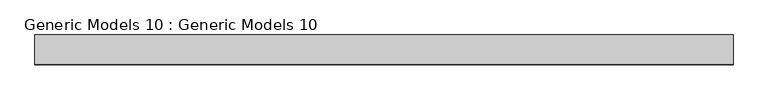
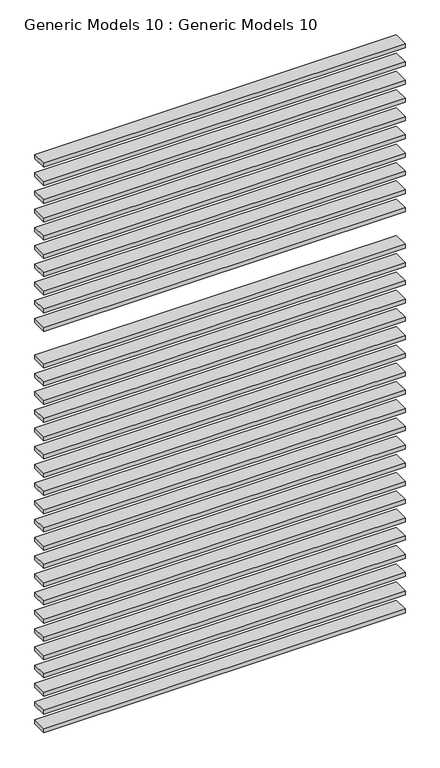
"""IFC4 building model written with IfcOpenShell, lengths in millimetres: proxy geometry, Generic Models 10 : Generic Models 10."""

from ifc_helpers import new_model, si_unit, frame, origin, place, context, project, spatial, polyline, outline, extrude, source, transform, mapped, element, save


def generic_models_10_generic_models_10_37b285cf(model_context):
    return source(origin(), model_context, "Body", "SweptSolid", [
        extrude(outline(polyline([(-8004.4916253, -6728.8336164), (-10858.4873516, -6728.8336164), (-10858.4873516, -6608.1640695), (-8004.4916253, -6608.1640695), (-8004.4916253, -6728.8336164)])), frame((0.0, 0.0, 3244.6584632), z_axis=(0.0, 0.0, 1.0), x_axis=(1.0, 0.0, 0.0)), (0.0, 0.0, 1.0), 33.1662923),
        extrude(outline(polyline([(-8004.4916253, -6728.8336164), (-10858.4873516, -6728.8336164), (-10858.4873516, -6608.1640695), (-8004.4916253, -6608.1640695), (-8004.4916253, -6728.8336164)])), frame((0.0, 0.0, 3397.0584632), z_axis=(0.0, 0.0, 1.0), x_axis=(1.0, 0.0, 0.0)), (0.0, 0.0, 1.0), 33.1662923),
        extrude(outline(polyline([(-8004.4916253, -6728.8336164), (-10858.4873516, -6728.8336164), (-10858.4873516, -6608.1640695), (-8004.4916253, -6608.1640695), (-8004.4916253, -6728.8336164)])), frame((0.0, 0.0, 3549.4584632), z_axis=(0.0, 0.0, 1.0), x_axis=(1.0, 0.0, 0.0)), (0.0, 0.0, 1.0), 33.1662923),
        extrude(outline(polyline([(-8004.4916253, -6728.8336164), (-10858.4873516, -6728.8336164), (-10858.4873516, -6608.1640695), (-8004.4916253, -6608.1640695), (-8004.4916253, -6728.8336164)])), frame((0.0, 0.0, 3701.8584632), z_axis=(0.0, 0.0, 1.0), x_axis=(1.0, 0.0, 0.0)), (0.0, 0.0, 1.0), 33.1662923),
        extrude(outline(polyline([(-8004.4916253, -6728.8336164), (-10858.4873516, -6728.8336164), (-10858.4873516, -6608.1640695), (-8004.4916253, -6608.1640695), (-8004.4916253, -6728.8336164)])), frame((0.0, 0.0, 3854.2584632), z_axis=(0.0, 0.0, 1.0), x_axis=(1.0, 0.0, 0.0)), (0.0, 0.0, 1.0), 33.1662923),
        extrude(outline(polyline([(-8004.4916253, -6728.8336164), (-10858.4873516, -6728.8336164), (-10858.4873516, -6608.1640695), (-8004.4916253, -6608.1640695), (-8004.4916253, -6728.8336164)])), frame((0.0, 0.0, 4006.6584632), z_axis=(0.0, 0.0, 1.0), x_axis=(1.0, 0.0, 0.0)), (0.0, 0.0, 1.0), 33.1662923),
        extrude(outline(polyline([(-8004.4916253, -6728.8336164), (-10858.4873516, -6728.8336164), (-10858.4873516, -6608.1640695), (-8004.4916253, -6608.1640695), (-8004.4916253, -6728.8336164)])), frame((0.0, 0.0, 4159.0584632), z_axis=(0.0, 0.0, 1.0), x_axis=(1.0, 0.0, 0.0)), (0.0, 0.0, 1.0), 33.1662923),
        extrude(outline(polyline([(-8004.4916253, -6728.8336164), (-10858.4873516, -6728.8336164), (-10858.4873516, -6608.1640695), (-8004.4916253, -6608.1640695), (-8004.4916253, -6728.8336164)])), frame((0.0, 0.0, 4311.4584632), z_axis=(0.0, 0.0, 1.0), x_axis=(1.0, 0.0, 0.0)), (0.0, 0.0, 1.0), 33.1662923),
        extrude(outline(polyline([(-8004.4916253, -6728.8336164), (-10858.4873516, -6728.8336164), (-10858.4873516, -6608.1640695), (-8004.4916253, -6608.1640695), (-8004.4916253, -6728.8336164)])), frame((0.0, 0.0, 4463.8584632), z_axis=(0.0, 0.0, 1.0), x_axis=(1.0, 0.0, 0.0)), (0.0, 0.0, 1.0), 33.1662923),
        extrude(outline(polyline([(-8004.4916253, -6728.8336164), (-10858.4873516, -6728.8336164), (-10858.4873516, -6608.1640695), (-8004.4916253, -6608.1640695), (-8004.4916253, -6728.8336164)])), frame((0.0, 0.0, 4616.2584632), z_axis=(0.0, 0.0, 1.0), x_axis=(1.0, 0.0, 0.0)), (0.0, 0.0, 1.0), 33.1662923),
        extrude(outline(polyline([(-8004.4916253, -6728.8336164), (-10858.4873516, -6728.8336164), (-10858.4873516, -6608.1640695), (-8004.4916253, -6608.1640695), (-8004.4916253, -6728.8336164)])), frame((0.0, 0.0, 4768.6584632), z_axis=(0.0, 0.0, 1.0), x_axis=(1.0, 0.0, 0.0)), (0.0, 0.0, 1.0), 33.1662923),
        extrude(outline(polyline([(-8004.4916253, -6728.8336164), (-10858.4873516, -6728.8336164), (-10858.4873516, -6608.1640695), (-8004.4916253, -6608.1640695), (-8004.4916253, -6728.8336164)])), frame((0.0, 0.0, 4921.0584632), z_axis=(0.0, 0.0, 1.0), x_axis=(1.0, 0.0, 0.0)), (0.0, 0.0, 1.0), 33.1662923),
        extrude(outline(polyline([(-8004.4916253, -6728.8336164), (-10858.4873516, -6728.8336164), (-10858.4873516, -6608.1640695), (-8004.4916253, -6608.1640695), (-8004.4916253, -6728.8336164)])), frame((0.0, 0.0, 5073.4584632), z_axis=(0.0, 0.0, 1.0), x_axis=(1.0, 0.0, 0.0)), (0.0, 0.0, 1.0), 33.1662923),
        extrude(outline(polyline([(-8004.4916253, -6728.8336164), (-10858.4873516, -6728.8336164), (-10858.4873516, -6608.1640695), (-8004.4916253, -6608.1640695), (-8004.4916253, -6728.8336164)])), frame((0.0, 0.0, 5225.8584632), z_axis=(0.0, 0.0, 1.0), x_axis=(1.0, 0.0, 0.0)), (0.0, 0.0, 1.0), 33.1662923),
        extrude(outline(polyline([(-8004.4916253, -6728.8336164), (-10858.4873516, -6728.8336164), (-10858.4873516, -6608.1640695), (-8004.4916253, -6608.1640695), (-8004.4916253, -6728.8336164)])), frame((0.0, 0.0, 5378.2584632), z_axis=(0.0, 0.0, 1.0), x_axis=(1.0, 0.0, 0.0)), (0.0, 0.0, 1.0), 33.1662923),
        extrude(outline(polyline([(-8004.4916253, -6728.8336164), (-10858.4873516, -6728.8336164), (-10858.4873516, -6608.1640695), (-8004.4916253, -6608.1640695), (-8004.4916253, -6728.8336164)])), frame((0.0, 0.0, 5530.6584632), z_axis=(0.0, 0.0, 1.0), x_axis=(1.0, 0.0, 0.0)), (0.0, 0.0, 1.0), 33.1662923),
        extrude(outline(polyline([(-8004.4916253, -6728.8336164), (-10858.4873516, -6728.8336164), (-10858.4873516, -6608.1640695), (-8004.4916253, -6608.1640695), (-8004.4916253, -6728.8336164)])), frame((0.0, 0.0, 5683.0584632), z_axis=(0.0, 0.0, 1.0), x_axis=(1.0, 0.0, 0.0)), (0.0, 0.0, 1.0), 33.1662923),
        extrude(outline(polyline([(-8004.4916253, -6728.8336164), (-10858.4873516, -6728.8336164), (-10858.4873516, -6608.1640695), (-8004.4916253, -6608.1640695), (-8004.4916253, -6728.8336164)])), frame((0.0, 0.0, 5835.4584632), z_axis=(0.0, 0.0, 1.0), x_axis=(1.0, 0.0, 0.0)), (0.0, 0.0, 1.0), 33.1662923),
        extrude(outline(polyline([(-8004.4916253, -6728.8336164), (-10858.4873516, -6728.8336164), (-10858.4873516, -6608.1640695), (-8004.4916253, -6608.1640695), (-8004.4916253, -6728.8336164)])), frame((0.0, 0.0, 5987.8584632), z_axis=(0.0, 0.0, 1.0), x_axis=(1.0, 0.0, 0.0)), (0.0, 0.0, 1.0), 33.1662923),
        extrude(outline(polyline([(-8004.4916253, -6728.8336164), (-10858.4873516, -6728.8336164), (-10858.4873516, -6608.1640695), (-8004.4916253, -6608.1640695), (-8004.4916253, -6728.8336164)])), frame((0.0, 0.0, 6140.2584632), z_axis=(0.0, 0.0, 1.0), x_axis=(1.0, 0.0, 0.0)), (0.0, 0.0, 1.0), 33.1662923),
        extrude(outline(polyline([(-8004.4916253, -6728.8336164), (-10858.4873516, -6728.8336164), (-10858.4873516, -6608.1640695), (-8004.4916253, -6608.1640695), (-8004.4916253, -6728.8336164)])), frame((0.0, 0.0, 6292.6584632), z_axis=(0.0, 0.0, 1.0), x_axis=(1.0, 0.0, 0.0)), (0.0, 0.0, 1.0), 33.1662923),
        extrude(outline(polyline([(-8004.4916253, -6728.8336164), (-10858.4873516, -6728.8336164), (-10858.4873516, -6608.1640695), (-8004.4916253, -6608.1640695), (-8004.4916253, -6728.8336164)])), frame((0.0, 0.0, 6597.4584632), z_axis=(0.0, 0.0, 1.0), x_axis=(1.0, 0.0, 0.0)), (0.0, 0.0, 1.0), 33.1662923),
        extrude(outline(polyline([(-8004.4916253, -6728.8336164), (-10858.4873516, -6728.8336164), (-10858.4873516, -6608.1640695), (-8004.4916253, -6608.1640695), (-8004.4916253, -6728.8336164)])), frame((0.0, 0.0, 6749.8584632), z_axis=(0.0, 0.0, 1.0), x_axis=(1.0, 0.0, 0.0)), (0.0, 0.0, 1.0), 33.1662923),
        extrude(outline(polyline([(-8004.4916253, -6728.8336164), (-10858.4873516, -6728.8336164), (-10858.4873516, -6608.1640695), (-8004.4916253, -6608.1640695), (-8004.4916253, -6728.8336164)])), frame((0.0, 0.0, 6902.2584632), z_axis=(0.0, 0.0, 1.0), x_axis=(1.0, 0.0, 0.0)), (0.0, 0.0, 1.0), 33.1662923),
        extrude(outline(polyline([(-8004.4916253, -6728.8336164), (-10858.4873516, -6728.8336164), (-10858.4873516, -6608.1640695), (-8004.4916253, -6608.1640695), (-8004.4916253, -6728.8336164)])), frame((0.0, 0.0, 7054.6584632), z_axis=(0.0, 0.0, 1.0), x_axis=(1.0, 0.0, 0.0)), (0.0, 0.0, 1.0), 33.1662923),
        extrude(outline(polyline([(-8004.4916253, -6728.8336164), (-10858.4873516, -6728.8336164), (-10858.4873516, -6608.1640695), (-8004.4916253, -6608.1640695), (-8004.4916253, -6728.8336164)])), frame((0.0, 0.0, 7207.0584632), z_axis=(0.0, 0.0, 1.0), x_axis=(1.0, 0.0, 0.0)), (0.0, 0.0, 1.0), 33.1662923),
        extrude(outline(polyline([(-8004.4916253, -6728.8336164), (-10858.4873516, -6728.8336164), (-10858.4873516, -6608.1640695), (-8004.4916253, -6608.1640695), (-8004.4916253, -6728.8336164)])), frame((0.0, 0.0, 7359.4584632), z_axis=(0.0, 0.0, 1.0), x_axis=(1.0, 0.0, 0.0)), (0.0, 0.0, 1.0), 33.1662923),
        extrude(outline(polyline([(-8004.4916253, -6728.8336164), (-10858.4873516, -6728.8336164), (-10858.4873516, -6608.1640695), (-8004.4916253, -6608.1640695), (-8004.4916253, -6728.8336164)])), frame((0.0, 0.0, 7511.8584632), z_axis=(0.0, 0.0, 1.0), x_axis=(1.0, 0.0, 0.0)), (0.0, 0.0, 1.0), 33.1662923),
        extrude(outline(polyline([(-8004.4916253, -6728.8336164), (-10858.4873516, -6728.8336164), (-10858.4873516, -6608.1640695), (-8004.4916253, -6608.1640695), (-8004.4916253, -6728.8336164)])), frame((0.0, 0.0, 7664.2584632), z_axis=(0.0, 0.0, 1.0), x_axis=(1.0, 0.0, 0.0)), (0.0, 0.0, 1.0), 33.1662923),
        extrude(outline(polyline([(-8004.4916253, -6728.8336164), (-10858.4873516, -6728.8336164), (-10858.4873516, -6608.1640695), (-8004.4916253, -6608.1640695), (-8004.4916253, -6728.8336164)])), frame((0.0, 0.0, 7816.6584632), z_axis=(0.0, 0.0, 1.0), x_axis=(1.0, 0.0, 0.0)), (0.0, 0.0, 1.0), 33.1662923),
        extrude(outline(polyline([(-8004.4916253, -6728.8336164), (-10858.4873516, -6728.8336164), (-10858.4873516, -6608.1640695), (-8004.4916253, -6608.1640695), (-8004.4916253, -6728.8336164)])), frame((0.0, 0.0, 7969.0584632), z_axis=(0.0, 0.0, 1.0), x_axis=(1.0, 0.0, 0.0)), (0.0, 0.0, 1.0), 33.1662923),
    ])


if __name__ == "__main__":
    model = new_model("IFC4")
    model_context = context("Model", 3, world=origin())
    ifc_project = project(units=[si_unit("LENGTHUNIT", "METRE", prefix="MILLI")], contexts=[model_context])
    site = spatial("IfcSite", under=ifc_project)
    building = spatial("IfcBuilding", under=site)
    placement = place(None, origin())
    generic_models_10_generic_models_10_shape = generic_models_10_generic_models_10_37b285cf(model_context)
    element("IfcBuildingElementProxy", 1, Name="Generic Models 10 : Generic Models 10", ObjectType="Generic Models 10 : Generic Models 10", at=placement, inside=building, context=model_context, shape_type="MappedRepresentation", body=[
        mapped(generic_models_10_generic_models_10_shape, transform((0.0, 0.0, 0.0), x_axis=(1.0, 0.0, 0.0), y_axis=(0.0, 1.0, 0.0), z_axis=(0.0, 0.0, 1.0))),
    ])
    save(model, "model.ifc")
